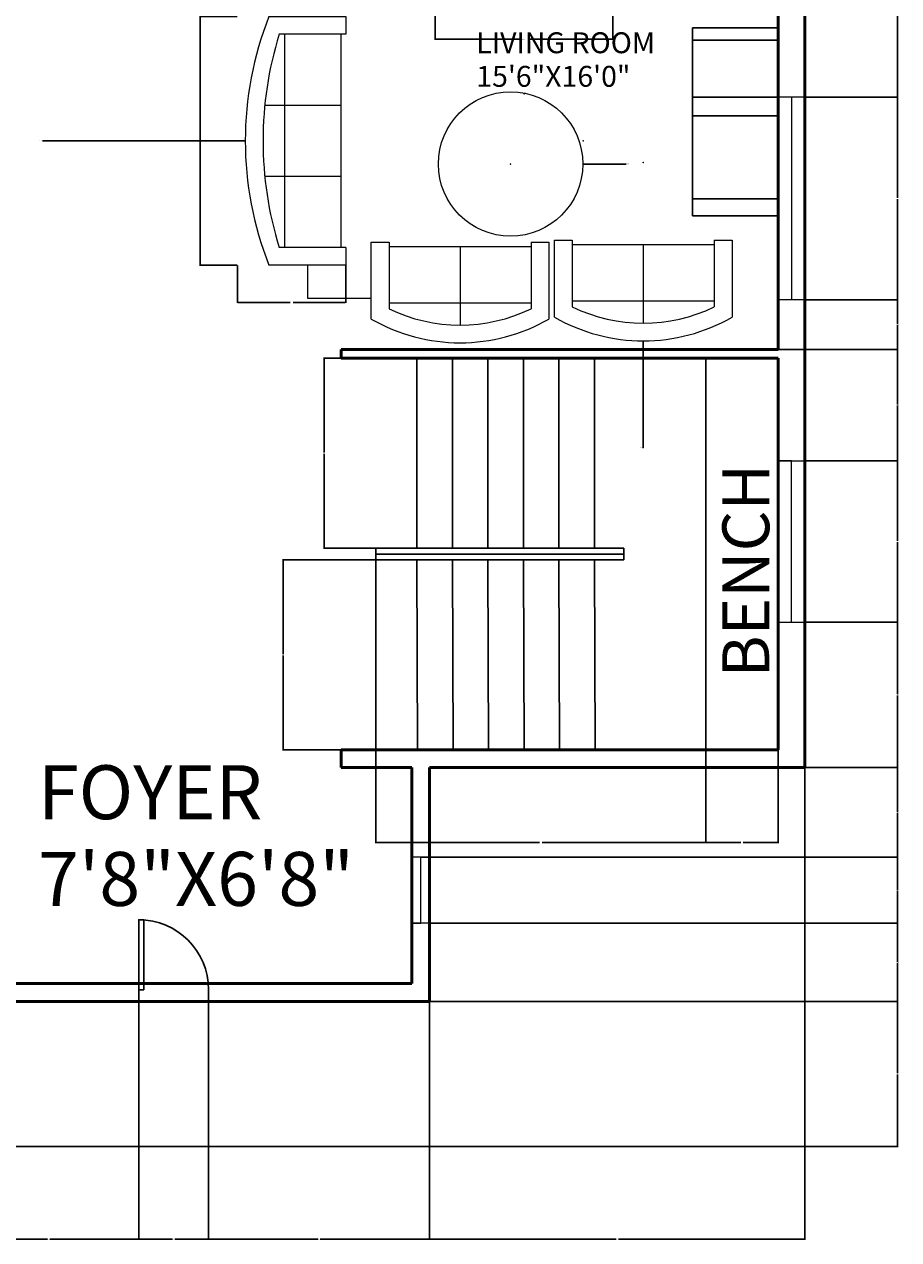
# Model space of a CAD drawing. Units: inches. Extents: x 2208 to 4689, y 1219 to 3512.
# Tile 3 of 5: x 2389 to 2685, y 1219 to 1629. Entities that reach past the tile are written whole.
import ezdxf

# ---------------------------------------------------------------- set-up
doc = ezdxf.new("R2010")
doc.units = ezdxf.units.IN
for name, color, linetype, lineweight in [('A-ANNO-DIMS', 2, 'Continuous', 18), ('A-ANNO-TEXT', 7, 'Continuous', 18), ('A-AREA-IDEN', 7, 'Continuous', 18), ('A-DOOR', 3, 'Continuous', 25), ('A-FLOR-CASE', 9, 'Continuous', 25), ('A-FLOR-STRS', 7, 'Continuous', 25), ('A-FURN', 8, 'Continuous', 18), ('A-GLAZ', 4, 'Continuous', 18), ('A-WALL', 7, 'Continuous', 50)]:
    doc.layers.add(name, color=color, linetype=linetype, lineweight=lineweight)
doc.styles.get("Standard").update_dxf_attribs({"font": 'arial.ttf'})
doc.dimstyles.get("Standard").update_dxf_attribs({"dimtxt": 0.18, "dimasz": 0.18, "dimexe": 0.18, "dimexo": 0.0625, "dimgap": 0.09, "dimtad": 0, "dimtih": 1, "dimtoh": 1, "dimdec": 4, "dimzin": 0, "dimdsep": 46, "dimtxsty": 'Standard', "dimcen": 0.09, "dimadec": 0, "dimazin": 0, "dimtfac": 1, "dimtdec": 4, "dimtofl": 0, "dimtmove": 0, "dimatfit": 3, "dimfxl": 1, "dimtolj": 1, "dimtzin": 0, "dimarcsym": 0})

# ---------------------------------------------------------------- blocks, each defined once
blk = doc.blocks.new('Sofa - Roundback 7 ft.')
for p, q in [((-12.00002, -32.4421), (-12.00003, -6.5971)), ((11.99997, -32.4421), (11.99998, -6.5971)), ((-36.000027, -34), (-36.000027, -11.4696)), ((35.99998, -34), (35.99998, -11.4696)), ((-35.999844, -13.3819), (35.9998, -13.3819)), ((-36.000027, -32.4421), (35.99998, -32.4421))]:
    blk.add_line(p, q)
for points in [[(-36.000027, -34), (-42.000027, -34), (-42.000027, -8)], [(41.99998, -8), (41.99998, -34), (35.99998, -34)]]:
    blk.add_lwpolyline(points)
for centre, radius, start, end in [((0, -114.25), 114.25, 68.43141, 111.5686), ((-0.00001, -127.1968), 121.1968, 72.72033, 107.2797)]:
    blk.add_arc(centre, radius, start, end)
blk = doc.blocks.new('Sofa - Roundback Loveseat 5 ft.')
for p, q in [((0, -32.44198), (0, -5.99998)), ((-24, -33.99998), (-24, -11.46958)), ((24.00004, -33.99998), (24.00004, -11.46958)), ((-23.9998, -13.38178), (23.99986, -13.38178)), ((-24, -32.44198), (24.00004, -32.44198))]:
    blk.add_line(p, q)
for points in [[(-24, -33.99998), (-30, -33.99998), (-30, -7.99998)], [(30.00004, -7.99998), (30.00004, -33.99998), (24.00004, -33.99998)]]:
    blk.add_lwpolyline(points)
for centre, radius, start, end in [((0, -60.24998), 60.24998, 60.13715, 119.8628), ((0, -61.38438), 55.38444, 64.32083, 115.6792)]:
    blk.add_arc(centre, radius, start, end)
blk = doc.blocks.new('*U15')
for p, q in [((0, 0), (0, -100)), ((600, 0), (600, -100))]:
    blk.add_line(p, q)
blk.add_lwpolyline([(0, 0), (0, 600), (43.75, 600), (43.75, 0)], close=True)
blk.add_arc((0, 0), 600, 0, 90)
blk = doc.blocks.new('*D18')
at = {"layer": 'A-ANNO-DIMS', "color": 0, "lineweight": -2, "transparency": 16777216}
for p, q in [((2528.21, 1633.35), (2528.21, 1624.23)), ((2588.21, 1633.35), (2588.21, 1624.23)), ((2528.39, 1624.41), (2556.98, 1624.41)), ((2588.03, 1624.41), (2559.43, 1624.41))]:
    blk.add_line(p, q, dxfattribs=at)
at = {"layer": 'A-ANNO-DIMS', "color": 0, "transparency": 16777216}
for points in [[(2528.39, 1624.44), (2528.39, 1624.38), (2528.21, 1624.41)], [(2588.03, 1624.44), (2588.03, 1624.38), (2588.21, 1624.41)]]:
    blk.add_solid(points, dxfattribs=at)
at = {"layer": 'Defpoints', "color": 0, "transparency": 16777216}
for p in [(2528.21, 1633.41), (2588.21, 1633.41), (2588.21, 1624.41)]:
    blk.add_point(p, dxfattribs=at)
at = {"layer": 'A-ANNO-DIMS', "color": 0, "transparency": 16777216, "insert": (2558.21, 1624.41), "char_height": 0.18, "attachment_point": 5}
blk.add_mtext('\\A1;LOVESEAT 60 TYP.', dxfattribs=at)
blk = doc.blocks.new('*D20')
at = {"layer": 'A-ANNO-DIMS', "color": 0, "lineweight": -2, "transparency": 16777216}
for p, q in [((2461.24, 1632.1), (2448.52, 1632.1)), ((2448.7, 1631.92), (2448.7, 1590.28)), ((2448.7, 1548.28), (2448.7, 1589.91)), ((2461.24, 1548.1), (2448.52, 1548.1))]:
    blk.add_line(p, q, dxfattribs=at)
at = {"layer": 'A-ANNO-DIMS', "color": 0, "transparency": 16777216}
for points in [[(2448.67, 1631.92), (2448.73, 1631.92), (2448.7, 1632.1)], [(2448.67, 1548.28), (2448.73, 1548.28), (2448.7, 1548.1)]]:
    blk.add_solid(points, dxfattribs=at)
at = {"layer": 'Defpoints', "color": 0, "transparency": 16777216}
for p in [(2448.7, 1632.1), (2461.3, 1632.1), (2461.3, 1548.1)]:
    blk.add_point(p, dxfattribs=at)
at = {"layer": 'A-ANNO-DIMS', "color": 0, "transparency": 16777216, "insert": (2448.7, 1590.1), "char_height": 0.18, "attachment_point": 5}
blk.add_mtext('\\A1;SOFA 84 TYP.', dxfattribs=at)
blk = doc.blocks.new('*D21')
at = {"layer": 'A-ANNO-DIMS', "color": 0, "lineweight": -2, "transparency": 16777216}
for p, q in [((2461.3, 1548.03), (2461.3, 1535.32)), ((2497.97, 1548.03), (2497.97, 1535.32)), ((2461.48, 1535.5), (2479.1, 1535.5)), ((2497.79, 1535.5), (2480.16, 1535.5))]:
    blk.add_line(p, q, dxfattribs=at)
at = {"layer": 'A-ANNO-DIMS', "color": 0, "transparency": 16777216}
for points in [[(2461.48, 1535.53), (2461.48, 1535.47), (2461.3, 1535.5)], [(2497.79, 1535.53), (2497.79, 1535.47), (2497.97, 1535.5)]]:
    blk.add_solid(points, dxfattribs=at)
at = {"layer": 'Defpoints', "color": 0, "transparency": 16777216}
for p in [(2461.3, 1548.1), (2497.97, 1548.1), (2461.3, 1535.5)]:
    blk.add_point(p, dxfattribs=at)
at = {"layer": 'A-ANNO-DIMS', "color": 0, "transparency": 16777216, "insert": (2479.63, 1535.5), "char_height": 0.18, "attachment_point": 5}
blk.add_mtext('\\A1;37 TYP.', dxfattribs=at)
blk = doc.blocks.new('*D50')
at = {"layer": 'A-ANNO-DIMS', "color": 0, "lineweight": -2, "transparency": 16777216}
for p, q in [((2367.11, 1299.29), (2367.11, 1218.83)), ((2427.95, 1299.29), (2427.95, 1218.83)), ((2367.29, 1219.01), (2397.14, 1219.01)), ((2427.77, 1219.01), (2397.93, 1219.01))]:
    blk.add_line(p, q, dxfattribs=at)
at = {"layer": 'A-ANNO-DIMS', "color": 0, "transparency": 16777216}
for points in [[(2367.29, 1219.04), (2367.29, 1218.98), (2367.11, 1219.01)], [(2427.77, 1219.04), (2427.77, 1218.98), (2427.95, 1219.01)]]:
    blk.add_solid(points, dxfattribs=at)
at = {"layer": 'Defpoints', "color": 0, "transparency": 16777216}
for p in [(2367.11, 1299.36), (2427.95, 1299.36), (2427.95, 1219.01)]:
    blk.add_point(p, dxfattribs=at)
at = {"layer": 'A-ANNO-DIMS', "color": 0, "transparency": 16777216, "insert": (2397.53, 1219.01), "char_height": 0.18, "attachment_point": 5}
blk.add_mtext('\\A1;60.84', dxfattribs=at)
blk = doc.blocks.new('*D51')
at = {"layer": 'A-ANNO-DIMS', "color": 0, "lineweight": -2, "transparency": 16777216}
for p, q in [((2427.95, 1299.29), (2427.95, 1218.83)), ((2451.57, 1299.29), (2451.57, 1218.83)), ((2428.13, 1219.01), (2439.37, 1219.01)), ((2451.39, 1219.01), (2440.16, 1219.01))]:
    blk.add_line(p, q, dxfattribs=at)
at = {"layer": 'A-ANNO-DIMS', "color": 0, "transparency": 16777216}
for points in [[(2428.13, 1219.04), (2428.13, 1218.98), (2427.95, 1219.01)], [(2451.39, 1219.04), (2451.39, 1218.98), (2451.57, 1219.01)]]:
    blk.add_solid(points, dxfattribs=at)
at = {"layer": 'Defpoints', "color": 0, "transparency": 16777216}
for p in [(2427.95, 1299.36), (2451.57, 1299.36), (2451.57, 1219.01)]:
    blk.add_point(p, dxfattribs=at)
at = {"layer": 'A-ANNO-DIMS', "color": 0, "transparency": 16777216, "insert": (2439.76, 1219.01), "char_height": 0.18, "attachment_point": 5}
blk.add_mtext('\\A1;23.62', dxfattribs=at)
blk = doc.blocks.new('*D52')
at = {"layer": 'A-ANNO-DIMS', "color": 0, "lineweight": -2, "transparency": 16777216}
for p, q in [((2451.57, 1299.29), (2451.57, 1218.83)), ((2526.29, 1299.29), (2526.29, 1218.83)), ((2451.75, 1219.01), (2488.56, 1219.01)), ((2526.11, 1219.01), (2489.31, 1219.01))]:
    blk.add_line(p, q, dxfattribs=at)
at = {"layer": 'A-ANNO-DIMS', "color": 0, "transparency": 16777216}
for points in [[(2451.75, 1219.04), (2451.75, 1218.98), (2451.57, 1219.01)], [(2526.11, 1219.04), (2526.11, 1218.98), (2526.29, 1219.01)]]:
    blk.add_solid(points, dxfattribs=at)
at = {"layer": 'Defpoints', "color": 0, "transparency": 16777216}
for p in [(2451.57, 1299.36), (2526.29, 1299.36), (2526.29, 1219.01)]:
    blk.add_point(p, dxfattribs=at)
at = {"layer": 'A-ANNO-DIMS', "color": 0, "transparency": 16777216, "insert": (2488.93, 1219.01), "char_height": 0.18, "attachment_point": 5}
blk.add_mtext('\\A1;74.71', dxfattribs=at)
blk = doc.blocks.new('*D53')
at = {"layer": 'A-ANNO-DIMS', "color": 0, "lineweight": -2, "transparency": 16777216}
for p, q in [((2526.29, 1378.29), (2526.29, 1218.83)), ((2653.1, 1378.29), (2653.1, 1218.83)), ((2526.47, 1219.01), (2589.31, 1219.01)), ((2652.92, 1219.01), (2590.08, 1219.01))]:
    blk.add_line(p, q, dxfattribs=at)
at = {"layer": 'A-ANNO-DIMS', "color": 0, "transparency": 16777216}
for points in [[(2526.47, 1219.04), (2526.47, 1218.98), (2526.29, 1219.01)], [(2652.92, 1219.04), (2652.92, 1218.98), (2653.1, 1219.01)]]:
    blk.add_solid(points, dxfattribs=at)
at = {"layer": 'Defpoints', "color": 0, "transparency": 16777216}
for p in [(2526.29, 1378.36), (2653.1, 1378.36), (2653.1, 1219.01)]:
    blk.add_point(p, dxfattribs=at)
at = {"layer": 'A-ANNO-DIMS', "color": 0, "transparency": 16777216, "insert": (2589.69, 1219.01), "char_height": 0.18, "attachment_point": 5}
blk.add_mtext('\\A1;126.8', dxfattribs=at)
blk = doc.blocks.new('*D54')
at = {"layer": 'A-ANNO-DIMS', "color": 0, "lineweight": -2, "transparency": 16777216}
for p, q in [((2367.18, 1299.36), (2684.63, 1299.36)), ((2684.45, 1299.18), (2684.45, 1275.04)), ((2684.45, 1250.54), (2684.45, 1274.67)), ((2367.18, 1250.36), (2684.63, 1250.36))]:
    blk.add_line(p, q, dxfattribs=at)
at = {"layer": 'A-ANNO-DIMS', "color": 0, "transparency": 16777216}
for points in [[(2684.42, 1299.18), (2684.48, 1299.18), (2684.45, 1299.36)], [(2684.42, 1250.54), (2684.48, 1250.54), (2684.45, 1250.36)]]:
    blk.add_solid(points, dxfattribs=at)
at = {"layer": 'Defpoints', "color": 0, "transparency": 16777216}
for p in [(2367.11, 1299.36), (2684.45, 1299.36), (2367.11, 1250.36)]:
    blk.add_point(p, dxfattribs=at)
at = {"layer": 'A-ANNO-DIMS', "color": 0, "transparency": 16777216, "insert": (2684.45, 1274.86), "char_height": 0.18, "attachment_point": 5}
blk.add_mtext('\\A1;49', dxfattribs=at)
blk = doc.blocks.new('*D55')
at = {"layer": 'A-ANNO-DIMS', "color": 0, "lineweight": -2, "transparency": 16777216}
for p, q in [((2526.35, 1325.74), (2684.63, 1325.74)), ((2684.45, 1325.56), (2684.45, 1312.73)), ((2684.45, 1299.54), (2684.45, 1312.37)), ((2526.35, 1299.36), (2684.63, 1299.36))]:
    blk.add_line(p, q, dxfattribs=at)
at = {"layer": 'A-ANNO-DIMS', "color": 0, "transparency": 16777216}
for points in [[(2684.42, 1325.56), (2684.48, 1325.56), (2684.45, 1325.74)], [(2684.42, 1299.54), (2684.48, 1299.54), (2684.45, 1299.36)]]:
    blk.add_solid(points, dxfattribs=at)
at = {"layer": 'Defpoints', "color": 0, "transparency": 16777216}
for p in [(2526.29, 1325.74), (2684.45, 1325.74), (2526.29, 1299.36)]:
    blk.add_point(p, dxfattribs=at)
at = {"layer": 'A-ANNO-DIMS', "color": 0, "transparency": 16777216, "insert": (2684.45, 1312.55), "char_height": 0.18, "attachment_point": 5}
blk.add_mtext('\\A1;26.39', dxfattribs=at)
blk = doc.blocks.new('*D56')
at = {"layer": 'A-ANNO-DIMS', "color": 0, "lineweight": -2, "transparency": 16777216}
for p, q in [((2526.35, 1348.03), (2684.63, 1348.03)), ((2684.45, 1347.85), (2684.45, 1337.07)), ((2684.45, 1325.92), (2684.45, 1336.71)), ((2526.35, 1325.74), (2684.63, 1325.74))]:
    blk.add_line(p, q, dxfattribs=at)
at = {"layer": 'A-ANNO-DIMS', "color": 0, "transparency": 16777216}
for points in [[(2684.42, 1347.85), (2684.48, 1347.85), (2684.45, 1348.03)], [(2684.42, 1325.92), (2684.48, 1325.92), (2684.45, 1325.74)]]:
    blk.add_solid(points, dxfattribs=at)
at = {"layer": 'Defpoints', "color": 0, "transparency": 16777216}
for p in [(2526.29, 1348.03), (2684.45, 1348.03), (2526.29, 1325.74)]:
    blk.add_point(p, dxfattribs=at)
at = {"layer": 'A-ANNO-DIMS', "color": 0, "transparency": 16777216, "insert": (2684.45, 1336.89), "char_height": 0.18, "attachment_point": 5}
blk.add_mtext('\\A1;22.29', dxfattribs=at)
blk = doc.blocks.new('*D57')
at = {"layer": 'A-ANNO-DIMS', "color": 0, "lineweight": -2, "transparency": 16777216}
for p, q in [((2526.35, 1378.36), (2684.63, 1378.36)), ((2684.45, 1378.18), (2684.45, 1363.38)), ((2684.45, 1348.21), (2684.45, 1363.01)), ((2526.35, 1348.03), (2684.63, 1348.03))]:
    blk.add_line(p, q, dxfattribs=at)
at = {"layer": 'A-ANNO-DIMS', "color": 0, "transparency": 16777216}
for points in [[(2684.42, 1378.18), (2684.48, 1378.18), (2684.45, 1378.36)], [(2684.42, 1348.21), (2684.48, 1348.21), (2684.45, 1348.03)]]:
    blk.add_solid(points, dxfattribs=at)
at = {"layer": 'Defpoints', "color": 0, "transparency": 16777216}
for p in [(2526.29, 1378.36), (2684.45, 1378.36), (2526.29, 1348.03)]:
    blk.add_point(p, dxfattribs=at)
at = {"layer": 'A-ANNO-DIMS', "color": 0, "transparency": 16777216, "insert": (2684.45, 1363.19), "char_height": 0.18, "attachment_point": 5}
blk.add_mtext('\\A1;30.323', dxfattribs=at)
blk = doc.blocks.new('*D58')
at = {"layer": 'A-ANNO-DIMS', "color": 0, "lineweight": -2, "transparency": 16777216}
for p, q in [((2653.16, 1427.49), (2684.63, 1427.49)), ((2684.45, 1427.31), (2684.45, 1403.11)), ((2684.45, 1378.54), (2684.45, 1402.74)), ((2653.16, 1378.36), (2684.63, 1378.36))]:
    blk.add_line(p, q, dxfattribs=at)
at = {"layer": 'A-ANNO-DIMS', "color": 0, "transparency": 16777216}
for points in [[(2684.42, 1427.31), (2684.48, 1427.31), (2684.45, 1427.49)], [(2684.42, 1378.54), (2684.48, 1378.54), (2684.45, 1378.36)]]:
    blk.add_solid(points, dxfattribs=at)
at = {"layer": 'Defpoints', "color": 0, "transparency": 16777216}
for p in [(2653.1, 1427.49), (2684.45, 1427.49), (2653.1, 1378.36)]:
    blk.add_point(p, dxfattribs=at)
at = {"layer": 'A-ANNO-DIMS', "color": 0, "transparency": 16777216, "insert": (2684.45, 1402.92), "char_height": 0.18, "attachment_point": 5}
blk.add_mtext('\\A1;49.14', dxfattribs=at)
blk = doc.blocks.new('*D59')
at = {"layer": 'A-ANNO-DIMS', "color": 0, "lineweight": -2, "transparency": 16777216}
for p, q in [((2653.16, 1481.97), (2684.63, 1481.97)), ((2684.45, 1481.79), (2684.45, 1454.91)), ((2684.45, 1427.67), (2684.45, 1454.55)), ((2653.16, 1427.49), (2684.63, 1427.49))]:
    blk.add_line(p, q, dxfattribs=at)
at = {"layer": 'A-ANNO-DIMS', "color": 0, "transparency": 16777216}
for points in [[(2684.42, 1481.79), (2684.48, 1481.79), (2684.45, 1481.97)], [(2684.42, 1427.67), (2684.48, 1427.67), (2684.45, 1427.49)]]:
    blk.add_solid(points, dxfattribs=at)
at = {"layer": 'Defpoints', "color": 0, "transparency": 16777216}
for p in [(2653.1, 1481.97), (2684.45, 1481.97), (2653.1, 1427.49)]:
    blk.add_point(p, dxfattribs=at)
at = {"layer": 'A-ANNO-DIMS', "color": 0, "transparency": 16777216, "insert": (2684.45, 1454.73), "char_height": 0.18, "attachment_point": 5}
blk.add_mtext('\\A1;54.47', dxfattribs=at)
blk = doc.blocks.new('*D60')
at = {"layer": 'A-ANNO-DIMS', "color": 0, "lineweight": -2, "transparency": 16777216}
for p, q in [((2644.16, 1519.65), (2684.63, 1519.65)), ((2684.45, 1519.47), (2684.45, 1500.99)), ((2684.45, 1482.15), (2684.45, 1500.63)), ((2653.16, 1481.97), (2684.63, 1481.97))]:
    blk.add_line(p, q, dxfattribs=at)
at = {"layer": 'A-ANNO-DIMS', "color": 0, "transparency": 16777216}
for points in [[(2684.42, 1519.47), (2684.48, 1519.47), (2684.45, 1519.65)], [(2684.42, 1482.15), (2684.48, 1482.15), (2684.45, 1481.97)]]:
    blk.add_solid(points, dxfattribs=at)
at = {"layer": 'Defpoints', "color": 0, "transparency": 16777216}
for p in [(2644.1, 1519.65), (2684.45, 1519.65), (2653.1, 1481.97)]:
    blk.add_point(p, dxfattribs=at)
at = {"layer": 'A-ANNO-DIMS', "color": 0, "transparency": 16777216, "insert": (2684.45, 1500.81), "char_height": 0.18, "attachment_point": 5}
blk.add_mtext('\\A1;37.68', dxfattribs=at)
blk = doc.blocks.new('*D61')
at = {"layer": 'A-ANNO-DIMS', "color": 0, "lineweight": -2, "transparency": 16777216}
for p, q in [((2653.16, 1536.41), (2684.63, 1536.41)), ((2684.45, 1536.23), (2684.45, 1528.21)), ((2684.45, 1519.83), (2684.45, 1527.85)), ((2644.16, 1519.65), (2684.63, 1519.65))]:
    blk.add_line(p, q, dxfattribs=at)
at = {"layer": 'A-ANNO-DIMS', "color": 0, "transparency": 16777216}
for points in [[(2684.42, 1536.23), (2684.48, 1536.23), (2684.45, 1536.41)], [(2684.42, 1519.83), (2684.48, 1519.83), (2684.45, 1519.65)]]:
    blk.add_solid(points, dxfattribs=at)
at = {"layer": 'Defpoints', "color": 0, "transparency": 16777216}
for p in [(2653.1, 1536.41), (2684.45, 1536.41), (2644.1, 1519.65)]:
    blk.add_point(p, dxfattribs=at)
at = {"layer": 'A-ANNO-DIMS', "color": 0, "transparency": 16777216, "insert": (2684.45, 1528.03), "char_height": 0.18, "attachment_point": 5}
blk.add_mtext('\\A1;16.765', dxfattribs=at)
blk = doc.blocks.new('*D62')
at = {"layer": 'A-ANNO-DIMS', "color": 0, "lineweight": -2, "transparency": 16777216}
for p, q in [((2653.16, 1604.85), (2684.63, 1604.85)), ((2684.45, 1604.67), (2684.45, 1570.81)), ((2684.45, 1536.59), (2684.45, 1570.45)), ((2653.16, 1536.41), (2684.63, 1536.41))]:
    blk.add_line(p, q, dxfattribs=at)
at = {"layer": 'A-ANNO-DIMS', "color": 0, "transparency": 16777216}
for points in [[(2684.42, 1604.67), (2684.48, 1604.67), (2684.45, 1604.85)], [(2684.42, 1536.59), (2684.48, 1536.59), (2684.45, 1536.41)]]:
    blk.add_solid(points, dxfattribs=at)
at = {"layer": 'Defpoints', "color": 0, "transparency": 16777216}
for p in [(2653.1, 1604.85), (2684.45, 1604.85), (2653.1, 1536.41)]:
    blk.add_point(p, dxfattribs=at)
at = {"layer": 'A-ANNO-DIMS', "color": 0, "transparency": 16777216, "insert": (2684.45, 1570.63), "char_height": 0.18, "attachment_point": 5}
blk.add_mtext('\\A1;68.43', dxfattribs=at)
blk = doc.blocks.new('*D63')
at = {"layer": 'A-ANNO-DIMS', "color": 0, "lineweight": -2, "transparency": 16777216}
for p, q in [((2644.16, 1674.36), (2684.63, 1674.36)), ((2684.45, 1674.18), (2684.45, 1639.78)), ((2684.45, 1605.03), (2684.45, 1639.42)), ((2653.16, 1604.85), (2684.63, 1604.85))]:
    blk.add_line(p, q, dxfattribs=at)
at = {"layer": 'A-ANNO-DIMS', "color": 0, "transparency": 16777216}
for points in [[(2684.42, 1674.18), (2684.48, 1674.18), (2684.45, 1674.36)], [(2684.42, 1605.03), (2684.48, 1605.03), (2684.45, 1604.85)]]:
    blk.add_solid(points, dxfattribs=at)
at = {"layer": 'Defpoints', "color": 0, "transparency": 16777216}
for p in [(2644.1, 1674.36), (2684.45, 1674.36), (2653.1, 1604.85)]:
    blk.add_point(p, dxfattribs=at)
at = {"layer": 'A-ANNO-DIMS', "color": 0, "transparency": 16777216, "insert": (2684.45, 1639.6), "char_height": 0.18, "attachment_point": 5}
blk.add_mtext('\\A1;69.51', dxfattribs=at)
blk = doc.blocks.new('*D70')
at = {"layer": 'A-ANNO-DIMS', "color": 0, "lineweight": -2, "transparency": 16777216}
for p, q in [((2619.61, 1384.29), (2619.61, 1352.83)), ((2644.1, 1384.29), (2644.1, 1352.83)), ((2619.79, 1353.01), (2631.46, 1353.01)), ((2643.92, 1353.01), (2632.25, 1353.01))]:
    blk.add_line(p, q, dxfattribs=at)
at = {"layer": 'A-ANNO-DIMS', "color": 0, "transparency": 16777216}
for points in [[(2619.79, 1353.04), (2619.79, 1352.98), (2619.61, 1353.01)], [(2643.92, 1353.04), (2643.92, 1352.98), (2644.1, 1353.01)]]:
    blk.add_solid(points, dxfattribs=at)
at = {"layer": 'Defpoints', "color": 0, "transparency": 16777216}
for p in [(2619.61, 1384.36), (2644.1, 1384.36), (2619.61, 1353.01)]:
    blk.add_point(p, dxfattribs=at)
at = {"layer": 'A-ANNO-DIMS', "color": 0, "transparency": 16777216, "insert": (2631.85, 1353.01), "char_height": 0.18, "attachment_point": 5}
blk.add_mtext('\\A1;24.49', dxfattribs=at)
blk = doc.blocks.new('*D71')
at = {"layer": 'A-ANNO-DIMS', "color": 0, "lineweight": -2, "transparency": 16777216}
for p, q in [((2508.13, 1384.29), (2508.13, 1352.83)), ((2619.61, 1384.29), (2619.61, 1352.83)), ((2508.31, 1353.01), (2563.42, 1353.01)), ((2619.43, 1353.01), (2564.33, 1353.01))]:
    blk.add_line(p, q, dxfattribs=at)
at = {"layer": 'A-ANNO-DIMS', "color": 0, "transparency": 16777216}
for points in [[(2508.31, 1353.04), (2508.31, 1352.98), (2508.13, 1353.01)], [(2619.43, 1353.04), (2619.43, 1352.98), (2619.61, 1353.01)]]:
    blk.add_solid(points, dxfattribs=at)
at = {"layer": 'Defpoints', "color": 0, "transparency": 16777216}
for p in [(2508.13, 1384.36), (2619.61, 1384.36), (2508.13, 1353.01)]:
    blk.add_point(p, dxfattribs=at)
at = {"layer": 'A-ANNO-DIMS', "color": 0, "transparency": 16777216, "insert": (2563.87, 1353.01), "char_height": 0.18, "attachment_point": 5}
blk.add_mtext('\\A1;111.47', dxfattribs=at)
blk = doc.blocks.new('*D72')
at = {"layer": 'A-ANNO-DIMS', "color": 0, "lineweight": -2, "transparency": 16777216}
for p, q in [((2508.07, 1448.5), (2476.6, 1448.5)), ((2476.78, 1448.32), (2476.78, 1416.61)), ((2476.78, 1384.54), (2476.78, 1416.25)), ((2508.07, 1384.36), (2476.6, 1384.36))]:
    blk.add_line(p, q, dxfattribs=at)
at = {"layer": 'A-ANNO-DIMS', "color": 0, "transparency": 16777216}
for points in [[(2476.75, 1448.32), (2476.81, 1448.32), (2476.78, 1448.5)], [(2476.75, 1384.54), (2476.81, 1384.54), (2476.78, 1384.36)]]:
    blk.add_solid(points, dxfattribs=at)
at = {"layer": 'Defpoints', "color": 0, "transparency": 16777216}
for p in [(2476.78, 1448.5), (2508.13, 1448.5), (2508.13, 1384.36)]:
    blk.add_point(p, dxfattribs=at)
at = {"layer": 'A-ANNO-DIMS', "color": 0, "transparency": 16777216, "insert": (2476.78, 1416.43), "char_height": 0.18, "attachment_point": 5}
blk.add_mtext('\\A1;64.15', dxfattribs=at)
blk = doc.blocks.new('*D73')
at = {"layer": 'A-ANNO-DIMS', "color": 0, "lineweight": -2, "transparency": 16777216}
for p, q in [((2521.92, 1516.65), (2490.45, 1516.65)), ((2490.63, 1516.47), (2490.63, 1484.76)), ((2490.63, 1452.68), (2490.63, 1484.39)), ((2521.92, 1452.5), (2490.45, 1452.5))]:
    blk.add_line(p, q, dxfattribs=at)
at = {"layer": 'A-ANNO-DIMS', "color": 0, "transparency": 16777216}
for points in [[(2490.6, 1516.47), (2490.66, 1516.47), (2490.63, 1516.65)], [(2490.6, 1452.68), (2490.66, 1452.68), (2490.63, 1452.5)]]:
    blk.add_solid(points, dxfattribs=at)
at = {"layer": 'Defpoints', "color": 0, "transparency": 16777216}
for p in [(2490.63, 1516.65), (2521.98, 1516.65), (2521.98, 1452.5)]:
    blk.add_point(p, dxfattribs=at)
at = {"layer": 'A-ANNO-DIMS', "color": 0, "transparency": 16777216, "insert": (2490.63, 1484.57), "char_height": 0.18, "attachment_point": 5}
blk.add_mtext('\\A1;64.15', dxfattribs=at)
blk = doc.blocks.new('*D74')
at = {"layer": 'A-ANNO-DIMS', "color": 0, "lineweight": -2, "transparency": 16777216}
for p, q in [((2553.55, 1582.26), (2553.73, 1582.26)), ((2553.64, 1582.17), (2553.64, 1582.35)), ((2592.67, 1582.26), (2578.22, 1582.26))]:
    blk.add_line(p, q, dxfattribs=at)
at = {"layer": 'A-ANNO-DIMS', "color": 0, "transparency": 16777216}
blk.add_solid([(2578.22, 1582.3), (2578.22, 1582.24), (2578.04, 1582.26)], dxfattribs=at)
at = {"layer": 'Defpoints', "color": 0, "transparency": 16777216}
for p in [(2529.25, 1582.26), (2578.04, 1582.26)]:
    blk.add_point(p, dxfattribs=at)
at = {"layer": 'A-ANNO-DIMS', "color": 0, "transparency": 16777216, "insert": (2593.16, 1582.26), "char_height": 0.18, "attachment_point": 5}
blk.add_mtext('\\A1;∅48.79', dxfattribs=at)
blk = doc.blocks.new('*D77')
at = {"layer": 'A-ANNO-DIMS', "color": 0, "lineweight": -2, "transparency": 16777216}
for p, q in [((2395.42, 1590.1), (2463.79, 1590.1)), ((2578.13, 1590.1), (2578.31, 1590.1)), ((2578.22, 1590.01), (2578.22, 1590.19))]:
    blk.add_line(p, q, dxfattribs=at)
at = {"layer": 'A-ANNO-DIMS', "color": 0, "transparency": 16777216}
blk.add_solid([(2463.79, 1590.13), (2463.79, 1590.07), (2463.97, 1590.1)], dxfattribs=at)
at = {"layer": 'Defpoints', "color": 0, "transparency": 16777216}
for p in [(2463.97, 1590.1), (2578.22, 1590.1)]:
    blk.add_point(p, dxfattribs=at)
at = {"layer": 'A-ANNO-DIMS', "color": 0, "transparency": 16777216, "insert": (2394.67, 1590.1), "char_height": 0.18, "attachment_point": 5}
blk.add_mtext('\\A1;3X R114.25', dxfattribs=at)
blk = doc.blocks.new('*D79')
at = {"layer": 'A-ANNO-DIMS', "color": 0, "lineweight": -2, "transparency": 16777216}
for p, q in [((2598.4, 1582.77), (2598.58, 1582.77)), ((2598.49, 1582.68), (2598.49, 1582.86)), ((2598.49, 1486.37), (2598.49, 1522.34)), ((2598.31, 1486.37), (2598.49, 1486.37))]:
    blk.add_line(p, q, dxfattribs=at)
at = {"layer": 'A-ANNO-DIMS', "color": 0, "transparency": 16777216}
blk.add_solid([(2598.46, 1522.34), (2598.52, 1522.34), (2598.49, 1522.52)], dxfattribs=at)
at = {"layer": 'Defpoints', "color": 0, "transparency": 16777216}
for p in [(2598.49, 1582.77), (2598.49, 1522.52)]:
    blk.add_point(p, dxfattribs=at)
at = {"layer": 'A-ANNO-DIMS', "color": 0, "transparency": 16777216, "insert": (2597.63, 1486.37), "char_height": 0.18, "attachment_point": 5}
blk.add_mtext('\\A1;3X R60.25', dxfattribs=at)
blk = doc.blocks.new('*D80')
at = {"layer": 'A-ANNO-DIMS', "color": 0, "lineweight": -2, "transparency": 16777216}
for p, q in [((2558.02, 1694.64), (2558.2, 1694.64)), ((2558.2, 1694.64), (2558.2, 1661.59)), ((2558.12, 1606.03), (2558.3, 1606.03)), ((2558.21, 1605.94), (2558.21, 1606.12))]:
    blk.add_line(p, q, dxfattribs=at)
at = {"layer": 'A-ANNO-DIMS', "color": 0, "transparency": 16777216}
blk.add_solid([(2558.23, 1661.59), (2558.17, 1661.59), (2558.2, 1661.41)], dxfattribs=at)
at = {"layer": 'Defpoints', "color": 0, "transparency": 16777216}
for p in [(2558.2, 1661.41), (2558.21, 1606.03)]:
    blk.add_point(p, dxfattribs=at)
at = {"layer": 'A-ANNO-DIMS', "color": 0, "transparency": 16777216, "insert": (2557.35, 1694.64), "char_height": 0.18, "attachment_point": 5}
blk.add_mtext('\\A1;3X R55.38', dxfattribs=at)

msp = doc.modelspace()

# ---------------------------------------------------------------- linework, layer by layer
at = {"layer": 'A-FLOR-CASE'}
for p, q in [((2615.1102, 1564.8103), (2615.1102, 1628.2276)), ((2615.1102, 1628.2276), (2644.0983, 1628.2276)), ((2615.1102, 1624.1336), (2644.0983, 1624.1336)), ((2644.0983, 1604.8466), (2615.1102, 1604.8466)), ((2615.1102, 1604.8466), (2644.0983, 1604.8466)), ((2644.0983, 1604.8466), (2644.0983, 1598.5118)), ((2644.0983, 1598.5118), (2615.1102, 1598.5118)), ((2644.0983, 1570.4831), (2615.1102, 1570.4831)), ((2644.0983, 1564.8103), (2615.1102, 1564.8103)), ((2619.6078, 1516.6482), (2619.6078, 1384.3551))]:
    msp.add_line(p, q, dxfattribs=at)
at = {"layer": 'A-FLOR-STRS'}
for p, q in [((2521.9815, 1452.5016), (2521.9815, 1516.6482)), ((2533.9815, 1452.5016), (2533.9815, 1516.6482)), ((2545.9815, 1452.5016), (2545.9815, 1516.6482)), ((2557.9815, 1452.5016), (2557.9815, 1516.6482)), ((2569.9815, 1452.5016), (2569.9815, 1516.6482)), ((2581.9815, 1452.5016), (2581.9815, 1516.6482)), ((2591.8918, 1452.5016), (2508.1341, 1452.5016)), ((2508.1341, 1452.5016), (2508.1341, 1448.5016)), ((2591.8918, 1450.5017), (2508.1341, 1450.5017)), ((2591.8918, 1452.5016), (2591.8918, 1448.5016)), ((2591.8918, 1448.5016), (2508.1341, 1448.5016)), ((2508.1341, 1448.5016), (2508.1341, 1384.3551)), ((2521.9819, 1448.3044), (2522.1928, 1384.1578)), ((2533.9818, 1448.3438), (2534.1927, 1384.1972)), ((2545.9817, 1448.3833), (2546.1927, 1384.2367)), ((2557.9817, 1448.4227), (2558.1926, 1384.2761)), ((2569.9816, 1448.4622), (2570.1925, 1384.3156)), ((2581.9815, 1448.5016), (2582.1925, 1384.3551))]:
    msp.add_line(p, q, dxfattribs=at)
at = {"layer": 'A-FURN'}
for p, q in [((2484.9651, 1548.0963), (2484.9651, 1536.9037)), ((2484.9651, 1536.9037), (2506.5717, 1536.9037))]:
    msp.add_line(p, q, dxfattribs=at)
msp.add_circle((2553.6425, 1582.2649), 24.3941, dxfattribs=at)
at = {"layer": 'A-GLAZ'}
for p, q in [((2653.0983, 1604.8466), (2644.0983, 1604.8466)), ((2648.5983, 1604.8466), (2648.5983, 1536.4132)), ((2653.0983, 1536.4132), (2644.0983, 1536.4132)), ((2648.5983, 1481.9684), (2644.0983, 1481.9684)), ((2644.0983, 1481.9684), (2653.0983, 1481.9684)), ((2648.5983, 1427.4946), (2648.5983, 1481.9684)), ((2644.0983, 1427.4946), (2653.0983, 1427.4946)), ((2526.2866, 1348.0319), (2520.2866, 1348.0319)), ((2523.2866, 1325.7429), (2523.2866, 1348.0319)), ((2523.2866, 1348.0319), (2526.2866, 1348.0319)), ((2526.2866, 1325.7429), (2520.2866, 1325.7429)), ((2520.2866, 1325.7429), (2523.2866, 1325.7429))]:
    msp.add_line(p, q, dxfattribs=at)
at = {"layer": 'A-WALL'}
for p, q in [((2653.0983, 1378.3551), (2653.0983, 1850.3551)), ((2644.0983, 1519.6482), (2644.0983, 1674.3551)), ((2496.4358, 1519.6482), (2520.2866, 1519.6482)), ((2496.4358, 1519.6482), (2496.4358, 1516.6482)), ((2520.2866, 1519.6482), (2644.0983, 1519.6482)), ((2496.4358, 1516.6482), (2520.2866, 1516.6482)), ((2520.2866, 1516.6482), (2644.0983, 1516.6482)), ((2644.0983, 1384.3551), (2644.0983, 1516.6482)), ((2496.4358, 1384.3551), (2496.4358, 1378.3551)), ((2496.4358, 1384.3551), (2520.2866, 1384.3551)), ((2520.2866, 1384.3551), (2644.0983, 1384.3551)), ((2496.4358, 1378.3551), (2520.2866, 1378.3551)), ((2520.2866, 1305.3551), (2520.2866, 1378.3551)), ((2526.2866, 1378.3551), (2644.0983, 1378.3551)), ((2526.2866, 1305.3551), (2526.2866, 1378.3551)), ((2644.0983, 1378.3551), (2653.0983, 1378.3551)), ((2520.2866, 1305.3551), (2520.2866, 1339.3551)), ((2367.1139, 1305.3551), (2520.2866, 1305.3551)), ((2526.2866, 1305.3551), (2526.2866, 1299.3551)), ((2367.1139, 1299.3551), (2526.2866, 1299.3551))]:
    msp.add_line(p, q, dxfattribs=at)

# ---------------------------------------------------------------- block references
at = {"layer": 'A-DOOR', "xscale": 0.0393700787401575, "yscale": 0.0393700787401575, "zscale": 0.0393700787401575}
msp.add_blockref('*U15', (2427.9528, 1303.2921), dxfattribs=at)
at = {"layer": 'A-FURN'}
for name, p, rotation in [('Sofa - Roundback 7 ft.', (2463.9651, 1590.0963), 90), ('Sofa - Roundback Loveseat 5 ft.', (2598.4921, 1522.5249), 180), ('Sofa - Roundback Loveseat 5 ft.', (2536.5718, 1521.8702), 180), ('Sofa - Roundback Loveseat 5 ft.', (2536.5718, 1521.8702), 180)]:
    msp.add_blockref(name, p, dxfattribs=dict(at, rotation=rotation))

# ---------------------------------------------------------------- texts
at = {"layer": 'A-ANNO-TEXT'}
msp.add_text('BENCH', height=15.85544, rotation=90, dxfattribs=at).set_placement((2641.0779, 1408.781))
at = {"layer": 'A-AREA-IDEN'}
for s, height, p in [('LIVING ROOM', 7.063632, (2542.0431, 1619.7081)), ('15\'6"X16\'0"', 7.063632, (2542.0431, 1608.361)), ('FOYER', 18.22124, (2393.9385, 1360.894)), ('7\'8"X6\'8"', 18.22124, (2393.9385, 1331.6232))]:
    msp.add_text(s, height=height, dxfattribs=at).set_placement(p)

# ---------------------------------------------------------------- dimensions: what is measured, and where the dimension line sits
at = {"layer": 'A-ANNO-DIMS'}
for center, mpoint, picture, middle in [((2558.2051, 1606.0251), (2558.205, 1661.4095), '*D80', (2557.3516, 1694.6402)), ((2578.2151, 1590.0963), (2463.9651, 1590.096), '*D77', (2395.4151, 1590.0958)), ((2598.4921, 1582.7749), (2598.49, 1522.5249), '*D79', (2597.6349, 1486.375))]:
    dim = msp.add_radius_dim(center=center, mpoint=mpoint, text='3X <>', dimstyle='Standard', override={"dimdec": 2, "dimlfac": 1, "dimrnd": 0, "dimzin": 0, "dimdsep": 46, "dimlunit": 2}, dxfattribs=at)
    dim.commit()
    dim.dimension.update_dxf_attribs({"geometry": picture, "text_midpoint": middle, "dimtype": 164})
for base, p1, p2, angle, override, picture, middle in [((2684.4483, 1674.3551), (2653.0983, 1604.8466), (2644.0983, 1674.3551), 90, {"dimdec": 2, "dimlfac": 1, "dimrnd": 0, "dimzin": 0, "dimdsep": 46, "dimlunit": 2}, '*D63', (2684.4483, 1639.6008)), ((2684.4483, 1604.8466), (2653.0983, 1536.4132), (2653.0983, 1604.8466), 90, {"dimdec": 2, "dimlfac": 1, "dimrnd": 0, "dimzin": 0, "dimdsep": 46, "dimlunit": 2}, '*D62', (2684.4483, 1570.6299)), ((2684.4483, 1536.4132), (2644.0983, 1519.6482), (2653.0983, 1536.4132), 90, {"dimdec": 3, "dimlfac": 1, "dimrnd": 0, "dimzin": 0, "dimdsep": 46, "dimlunit": 2}, '*D61', (2684.4483, 1528.0307)), ((2684.4483, 1519.6482), (2653.0983, 1481.9684), (2644.0983, 1519.6482), 90, {"dimdec": 2, "dimlfac": 1, "dimrnd": 0, "dimzin": 0, "dimdsep": 46, "dimlunit": 2}, '*D60', (2684.4483, 1500.8083)), ((2490.6315, 1516.6482), (2521.9815, 1452.5016), (2521.9815, 1516.6482), 90, {"dimdec": 2, "dimlfac": 1, "dimrnd": 0, "dimzin": 0, "dimdsep": 46, "dimlunit": 2}, '*D73', (2490.6315, 1484.5749)), ((2684.4483, 1481.9684), (2653.0983, 1427.4946), (2653.0983, 1481.9684), 90, {"dimdec": 2, "dimlfac": 1, "dimrnd": 0, "dimzin": 0, "dimdsep": 46, "dimlunit": 2}, '*D59', (2684.4483, 1454.7315)), ((2476.7841, 1448.5016), (2508.1341, 1384.3551), (2508.1341, 1448.5016), 90, {"dimdec": 2, "dimlfac": 1, "dimrnd": 0, "dimzin": 0, "dimdsep": 46, "dimlunit": 2}, '*D72', (2476.7841, 1416.4284)), ((2684.4483, 1427.4946), (2653.0983, 1378.3551), (2653.0983, 1427.4946), 90, {"dimdec": 2, "dimlfac": 1, "dimrnd": 0, "dimzin": 0, "dimdsep": 46, "dimlunit": 2}, '*D58', (2684.4483, 1402.9248)), ((2508.1341, 1353.0051), (2619.6078, 1384.3551), (2508.1341, 1384.3551), 180, {"dimdec": 2, "dimlfac": 1, "dimrnd": 0, "dimzin": 0, "dimdsep": 46, "dimlunit": 2}, '*D71', (2563.8709, 1353.0051)), ((2619.6078, 1353.0051), (2644.0983, 1384.3551), (2619.6078, 1384.3551), 180, {"dimdec": 2, "dimlfac": 1, "dimrnd": 0, "dimzin": 0, "dimdsep": 46, "dimlunit": 2}, '*D70', (2631.853, 1353.0051)), ((2684.4483, 1378.3551), (2526.2866, 1348.0319), (2526.2866, 1378.3551), 90, {"dimdec": 3, "dimlfac": 1, "dimrnd": 0, "dimzin": 0, "dimdsep": 46, "dimlunit": 2}, '*D57', (2684.4483, 1363.1935)), ((2684.4483, 1348.0319), (2526.2866, 1325.7429), (2526.2866, 1348.0319), 90, {"dimdec": 2, "dimlfac": 1, "dimrnd": 0, "dimzin": 0, "dimdsep": 46, "dimlunit": 2}, '*D56', (2684.4483, 1336.8874)), ((2684.4483, 1325.7429), (2526.2866, 1299.3551), (2526.2866, 1325.7429), 90, {"dimdec": 2, "dimlfac": 1, "dimrnd": 0, "dimzin": 0, "dimdsep": 46, "dimlunit": 2}, '*D55', (2684.4483, 1312.549)), ((2684.4483, 1299.3551), (2367.1139, 1250.3551), (2367.1139, 1299.3551), 90, {"dimdec": 0, "dimlfac": 1, "dimrnd": 0, "dimzin": 0, "dimdsep": 46, "dimlunit": 2}, '*D54', (2684.4483, 1274.8551))]:
    dim = msp.add_linear_dim(base=base, p1=p1, p2=p2, angle=angle, dimstyle='Standard', override=override, dxfattribs=at)
    dim.commit()
    dim.dimension.update_dxf_attribs({"geometry": picture, "text_midpoint": middle})
for base, p1, p2, angle, text, picture, middle in [((2448.6984, 1632.0963), (2461.2984, 1548.0963), (2461.2984, 1632.0963), 90, 'SOFA <> TYP.', '*D20', (2448.6984, 1590.0963)), ((2461.2984, 1535.4963), (2497.9651, 1548.0963), (2461.2984, 1548.0963), 180, '<> TYP.', '*D21', (2479.6318, 1535.4963))]:
    dim = msp.add_linear_dim(base=base, p1=p1, p2=p2, angle=angle, text=text, dimstyle='Standard', override={"dimdec": 0, "dimlfac": 1, "dimrnd": 0, "dimzin": 0, "dimdsep": 46, "dimlunit": 2}, dxfattribs=at)
    dim.commit()
    dim.dimension.update_dxf_attribs({"geometry": picture, "text_midpoint": middle})
dim = msp.add_linear_dim(base=(2588.2052, 1624.4095), p1=(2528.2051, 1633.4095), p2=(2588.2052, 1633.4095), text='LOVESEAT <> TYP.', dimstyle='Standard', override={"dimdec": 0, "dimlfac": 1, "dimrnd": 0, "dimzin": 0, "dimdsep": 46, "dimlunit": 2}, dxfattribs=at)
dim.commit()
dim.dimension.update_dxf_attribs({"geometry": '*D18', "text_midpoint": (2558.2052, 1624.4095)})
dim = msp.add_diameter_dim_2p(p1=(2529.2484, 1582.2648), p2=(2578.0366, 1582.265), dimstyle='Standard', override={"dimdec": 2, "dimlfac": 1, "dimrnd": 0, "dimzin": 0, "dimdsep": 46, "dimlunit": 2}, dxfattribs=at)
dim.commit()
dim.dimension.update_dxf_attribs({"geometry": '*D74', "text_midpoint": (2592.6731, 1582.2651), "dimtype": 163})
for base, p1, p2, override, picture, middle in [((2653.0983, 1219.0051), (2526.2866, 1378.3551), (2653.0983, 1378.3551), {"dimdec": 1, "dimlfac": 1, "dimrnd": 0, "dimzin": 0, "dimdsep": 46, "dimlunit": 2}, '*D53', (2589.6925, 1219.0051)), ((2427.9528, 1219.0051), (2367.1139, 1299.3551), (2427.9528, 1299.3551), {"dimdec": 2, "dimlfac": 1, "dimrnd": 0, "dimzin": 0, "dimdsep": 46, "dimlunit": 2}, '*D50', (2397.5333, 1219.0051)), ((2451.5748, 1219.0051), (2427.9528, 1299.3551), (2451.5748, 1299.3551), {"dimdec": 2, "dimlfac": 1, "dimrnd": 0, "dimzin": 0, "dimdsep": 46, "dimlunit": 2}, '*D51', (2439.7638, 1219.0051)), ((2526.2866, 1219.0051), (2451.5748, 1299.3551), (2526.2866, 1299.3551), {"dimdec": 2, "dimlfac": 1, "dimrnd": 0, "dimzin": 0, "dimdsep": 46, "dimlunit": 2}, '*D52', (2488.9307, 1219.0051))]:
    dim = msp.add_linear_dim(base=base, p1=p1, p2=p2, dimstyle='Standard', override=override, dxfattribs=at)
    dim.commit()
    dim.dimension.update_dxf_attribs({"geometry": picture, "text_midpoint": middle})

doc.saveas('drawing.dxf')
